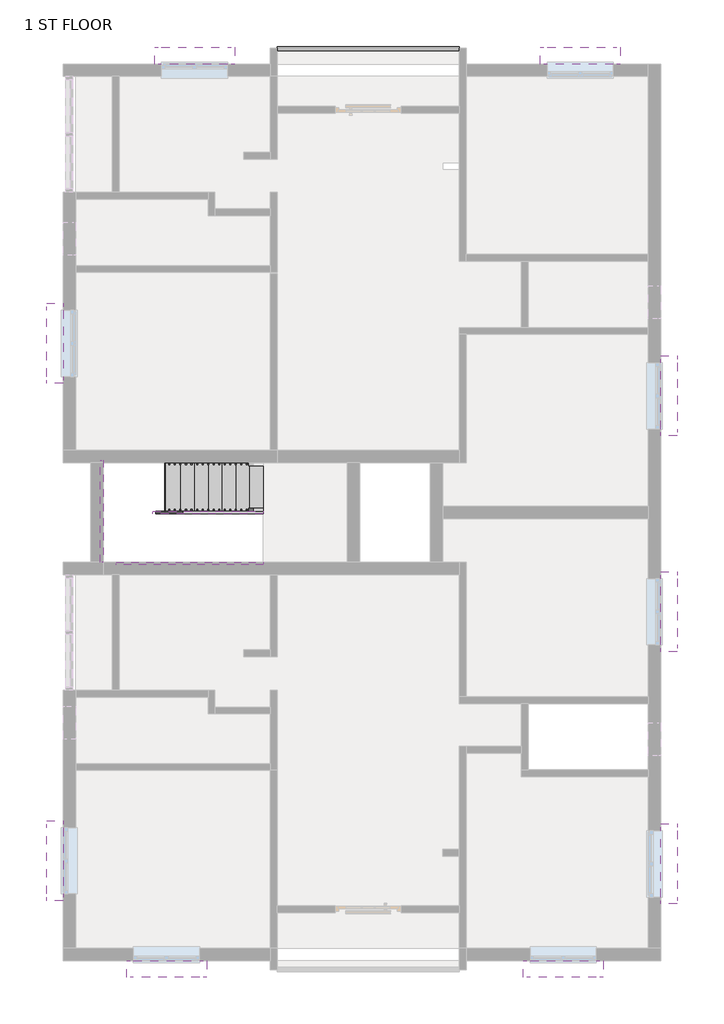
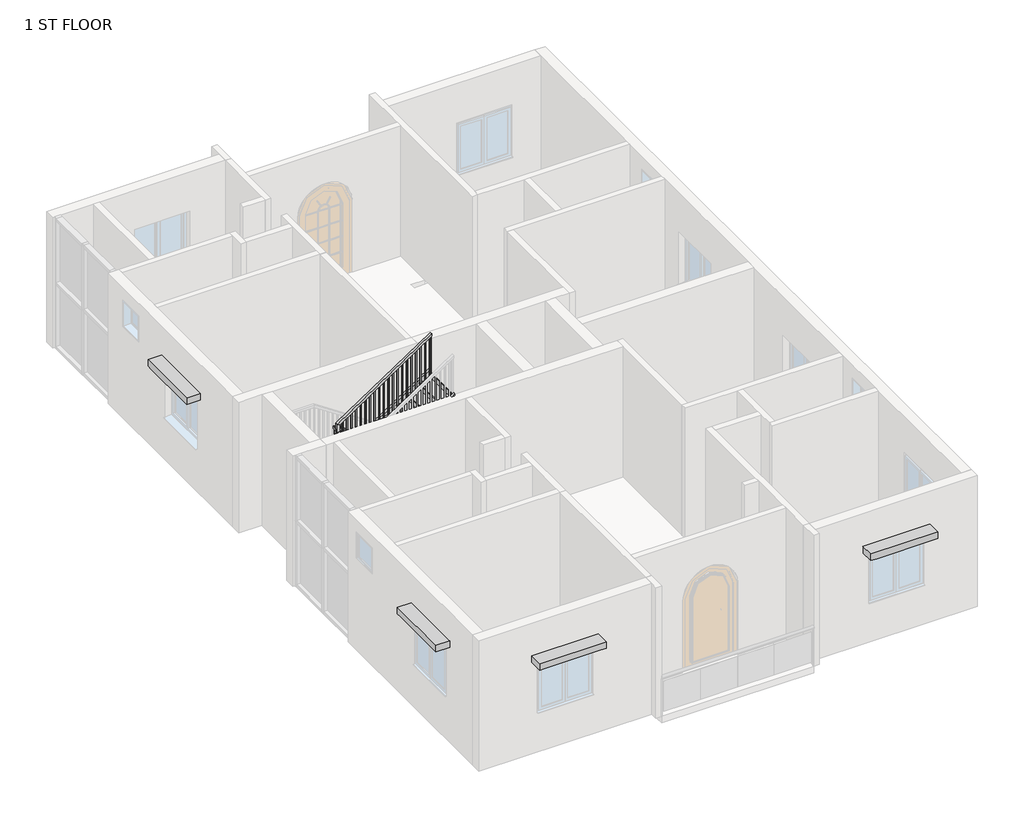
# One storey, part 4 of 4: 9 proxies, 5 members, 2 railings, 1 stair flight.
"""IFC4 building model written with IfcOpenShell, lengths in millimetres."""

from ifc_helpers import new_model, si_unit, point, frame, origin, place, context, project, spatial, polyline, ellipse_curve, trimmed, outline, extrude, faceted_brep, transform, mapped, element, save
from ifc_brep_helpers import plane_surface, extruded_surface, advanced_brep
from components import generic_models_11_generic_models_11_d301a5e8, generic_models_21_generic_models_21_87948dc1, generic_models_36_generic_models_36_9c63594f, generic_models_1_generic_models_1_fbb7ad13, stair_flight_02872950

model = new_model("IFC4")

# Units and contexts
model_context = context("Model", 3, world=origin())
ifc_project = project(units=[si_unit("LENGTHUNIT", "METRE", prefix="MILLI")], contexts=[model_context])

# Site, building, storey
site = spatial("IfcSite", under=ifc_project)
building = spatial("IfcBuilding", under=site)
storey = spatial("IfcBuildingStorey", under=building, Name="1 ST FLOOR", Elevation=6096.0)

# Proxies
placement = place(None, origin())
generic_models_11_generic_models_11_shape = generic_models_11_generic_models_11_d301a5e8(model_context)
element("IfcBuildingElementProxy", 1, Name="Generic Models 17 : Generic Models 11", ObjectType="Generic Models 17 : Generic Models 11", at=placement, inside=storey, context=model_context, shape_type="MappedRepresentation", body=[
    mapped(generic_models_11_generic_models_11_shape, transform((0.0, 0.0, -9144.0), x_axis=(1.0, 0.0, 0.0), y_axis=(0.0, 1.0, 0.0), z_axis=(0.0, 0.0, 1.0))),
])
element("IfcBuildingElementProxy", 2, Name="Generic Models 18 : Generic Models 11", ObjectType="Generic Models 18 : Generic Models 11", at=placement, inside=storey, context=model_context, shape_type="MappedRepresentation", body=[
    mapped(generic_models_11_generic_models_11_shape, transform((-7101.0359618, 0.0, -9144.0), x_axis=(1.0, 0.0, 0.0), y_axis=(0.0, 1.0, 0.0), z_axis=(0.0, 0.0, 1.0))),
])
generic_models_21_generic_models_21_shape = generic_models_21_generic_models_21_87948dc1(model_context)
element("IfcBuildingElementProxy", 3, Name="Generic Models 30 : Generic Models 21", ObjectType="Generic Models 30 : Generic Models 21", at=placement, inside=storey, context=model_context, shape_type="MappedRepresentation", body=[
    mapped(generic_models_21_generic_models_21_shape, transform((0.0, 0.0, -9144.0), x_axis=(1.0, 0.0, 0.0), y_axis=(0.0, 1.0, 0.0), z_axis=(0.0, 0.0, 1.0))),
])
element("IfcBuildingElementProxy", 4, Name="Generic Models 31 : Generic Models 21", ObjectType="Generic Models 31 : Generic Models 21", at=placement, inside=storey, context=model_context, shape_type="MappedRepresentation", body=[
    mapped(generic_models_21_generic_models_21_shape, transform((0.0, 4641.85, -9229.6), x_axis=(1.0, 0.0, 0.0), y_axis=(0.0, 1.0, 0.0), z_axis=(0.0, 0.0, 1.0))),
])
element("IfcBuildingElementProxy", 5, Name="Generic Models 32 : Generic Models 21", ObjectType="Generic Models 32 : Generic Models 21", at=placement, inside=storey, context=model_context, shape_type="MappedRepresentation", body=[
    mapped(generic_models_21_generic_models_21_shape, transform((0.0, 8616.95, -9229.6), x_axis=(1.0, 0.0, 0.0), y_axis=(0.0, 1.0, 0.0), z_axis=(0.0, 0.0, 1.0))),
])
generic_models_36_generic_models_36_shape = generic_models_36_generic_models_36_9c63594f(model_context)
element("IfcBuildingElementProxy", 6, Name="Generic Models 42 : Generic Models 36", ObjectType="Generic Models 42 : Generic Models 36", at=placement, inside=storey, context=model_context, shape_type="MappedRepresentation", body=[
    mapped(generic_models_36_generic_models_36_shape, transform((0.0, 0.0, -9144.0), x_axis=(1.0, 0.0, 0.0), y_axis=(0.0, 1.0, 0.0), z_axis=(0.0, 0.0, 1.0))),
])
element("IfcBuildingElementProxy", 7, Name="Generic Models 43 : Generic Models 36", ObjectType="Generic Models 43 : Generic Models 36", at=placement, inside=storey, context=model_context, shape_type="MappedRepresentation", body=[
    mapped(generic_models_36_generic_models_36_shape, transform((0.0, -9525.0, -9144.0), x_axis=(1.0, 0.0, 0.0), y_axis=(0.0, 1.0, 0.0), z_axis=(0.0, 0.0, 1.0))),
])
generic_models_1_generic_models_1_shape = generic_models_1_generic_models_1_fbb7ad13(model_context)
element("IfcBuildingElementProxy", 8, Name="Generic Models 7 : Generic Models 1", ObjectType="Generic Models 7 : Generic Models 1", at=placement, inside=storey, context=model_context, shape_type="MappedRepresentation", body=[
    mapped(generic_models_1_generic_models_1_shape, transform((0.0, 0.0, -9144.0), x_axis=(1.0, 0.0, 0.0), y_axis=(0.0, 1.0, 0.0), z_axis=(0.0, 0.0, 1.0))),
])
element("IfcBuildingElementProxy", 9, Name="Generic Models 8 : Generic Models 1", ObjectType="Generic Models 8 : Generic Models 1", at=placement, inside=storey, context=model_context, shape_type="MappedRepresentation", body=[
    mapped(generic_models_1_generic_models_1_shape, transform((7304.0875, 0.0, -9144.0), x_axis=(1.0, 0.0, 0.0), y_axis=(0.0, 1.0, 0.0), z_axis=(0.0, 0.0, 1.0))),
])

# Members
element("IfcMember", 10, ObjectType="Stringer - 2\" Width", at=placement, inside=storey, context=model_context, shape_type="SweptSolid", body=[
    extrude(outline(polyline([(6096.0, -2748.0012202), (6314.0398409, -2748.0012202), (7634.8398409, -4729.2012202), (7268.5158313, -4729.2012202), (6096.0, -2970.4274732), (6096.0, -2748.0012202)])), frame((0.0, 4990.8309003, 0.0), z_axis=(0.0, 1.0, 0.0), x_axis=(0.0, 0.0, 1.0)), (0.0, 0.0, 1.0), 50.8),
])
element("IfcMember", 11, ObjectType="Stringer - 2\" Width", at=placement, inside=storey, context=model_context, shape_type="SweptSolid", body=[
    extrude(outline(polyline([(7838.0398409, -4780.0012202), (7471.7158313, -4780.0012202), (8826.382498, -2748.0012202), (9192.7065076, -2748.0012202), (7838.0398409, -4780.0012202)])), frame((0.0, 4990.8309003, 0.0), z_axis=(0.0, 1.0, 0.0), x_axis=(0.0, 0.0, 1.0)), (0.0, 0.0, 1.0), 50.8),
])
element("IfcMember", 12, ObjectType="Stringer - 2\" Width", at=placement, inside=storey, context=model_context, shape_type="SweptSolid", body=[
    extrude(outline(polyline([(6096.0, -2748.0012202), (6314.0398409, -2748.0012202), (7696.2, -4821.2414588), (7696.2, -5370.7274732), (6096.0, -2970.4274732), (6096.0, -2748.0012202)])), frame((0.0, 5930.6309003, 0.0), z_axis=(0.0, 1.0, 0.0), x_axis=(0.0, 0.0, 1.0)), (0.0, 0.0, 1.0), 50.8),
])
element("IfcMember", 13, ObjectType="Stringer - 2\" Width", at=placement, inside=storey, context=model_context, shape_type="SweptSolid", body=[
    extrude(outline(polyline([(-5745.2012202, 5981.4309003), (-5694.4012202, 5981.4309003), (-5694.4012202, 4101.8309003), (-5745.2012202, 4101.8309003), (-5745.2012202, 5981.4309003)])), frame((0.0, 0.0, 7391.4), z_axis=(0.0, 0.0, 1.0), x_axis=(1.0, 0.0, 0.0)), (0.0, 0.0, 1.0), 304.8),
])
element("IfcMember", 14, ObjectType="Stringer - 2\" Width", at=placement, inside=storey, context=model_context, shape_type="SweptSolid", body=[
    extrude(outline(polyline([(7391.4, -4900.4749672), (8826.382498, -2748.0012202), (9192.7065076, -2748.0012202), (7391.4, -5449.9609815), (7391.4, -4900.4749672)])), frame((0.0, 4051.0309003, 0.0), z_axis=(0.0, 1.0, 0.0), x_axis=(0.0, 0.0, 1.0)), (0.0, 0.0, 1.0), 50.8),
])

# Railings
element("IfcRailing", 15, ObjectType="Glass Panel - Bottom Fill 2", at=placement, inside=storey, context=model_context, shape_type="SolidModel", body=[
    advanced_brep(
    [(-2494.0012202, 13593.7910566, 7010.4), (-2494.0012202, 13517.5910566, 7010.4), (858.7987798, 13593.7910566, 7010.4), (858.7987798, 13517.5910566, 7010.4)],
    [
        (0, 1, ellipse_curve(frame((-2494.0012202, 13555.6910566, 7010.4), z_axis=(-1.0, 0.0, 0.0), x_axis=(0.0, -1.0, 0.0)), 38.1, 28.575)),
        (1, 0, ellipse_curve(frame((-2494.0012202, 13555.6910566, 7010.4), z_axis=(-1.0, 0.0, 0.0), x_axis=(0.0, -1.0, 0.0)), 38.1, 28.575)),
        (2, 3, ellipse_curve(frame((858.7987798, 13555.6910566, 7010.4), z_axis=(1.0, 0.0, 0.0), x_axis=(0.0, -1.0, 0.0)), 38.1, 28.575)),
        (3, 2, ellipse_curve(frame((858.7987798, 13555.6910566, 7010.4), z_axis=(1.0, 0.0, 0.0), x_axis=(0.0, -1.0, 0.0)), 38.1, 28.575)),
        (0, 2),
        (3, 1),
    ],
    [
        plane_surface(frame((-2494.0012202, 13555.6910566, 7010.4), z_axis=(-1.0, 0.0, 0.0), x_axis=(0.0, 1.0, 0.0))),
        plane_surface(frame((858.7987798, 13555.6910566, 7010.4), z_axis=(1.0, 0.0, 0.0), x_axis=(0.0, 1.0, 0.0))),
        extruded_surface(trimmed(ellipse_curve(frame((858.7987798, 13555.6910566, 7010.4), z_axis=(-1.0, 0.0, 0.0), x_axis=(0.0, -1.0, 0.0)), 38.1, 28.575), [point((858.7987798, 13593.7910566, 7010.4))], [point((858.7987798, 13517.5910566, 7010.4))], True, "CARTESIAN"), (-3352.7999999999997, 0.0, 0.0), 3352.7999999999997),
        extruded_surface(trimmed(ellipse_curve(frame((858.7987798, 13555.6910566, 7010.4), z_axis=(-1.0, 0.0, 0.0), x_axis=(0.0, -1.0, 0.0)), 38.1, 28.575), [point((858.7987798, 13517.5910566, 7010.4))], [point((858.7987798, 13593.7910566, 7010.4))], True, "CARTESIAN"), (-3352.7999999999997, 0.0, 0.0), 3352.7999999999997),
    ],
    [
        (0, [[1, 2]]),
        (1, [[3, 4]]),
        (2, [[-1, 5, -4, 6]]),
        (3, [[-2, -6, -3, -5]]),
    ],
),
    extrude(outline(polyline([(-4.8012202, 13562.2262136), (807.9987798, 13562.2262136), (807.9987798, 13555.8762136), (-4.8012202, 13555.8762136), (-4.8012202, 13562.2262136)])), frame((0.0, 0.0, 6197.6), z_axis=(0.0, 0.0, 1.0), x_axis=(1.0, 0.0, 0.0)), (0.0, 0.0, 1.0), 711.2),
    extrude(outline(polyline([(-817.6012202, 13562.2262136), (-4.8012202, 13562.2262136), (-4.8012202, 13555.8762136), (-817.6012202, 13555.8762136), (-817.6012202, 13562.2262136)])), frame((0.0, 0.0, 6197.6), z_axis=(0.0, 0.0, 1.0), x_axis=(1.0, 0.0, 0.0)), (0.0, 0.0, 1.0), 711.2),
    extrude(outline(polyline([(-1630.4012202, 13562.2262136), (-817.6012202, 13562.2262136), (-817.6012202, 13555.8762136), (-1630.4012202, 13555.8762136), (-1630.4012202, 13562.2262136)])), frame((0.0, 0.0, 6197.6), z_axis=(0.0, 0.0, 1.0), x_axis=(1.0, 0.0, 0.0)), (0.0, 0.0, 1.0), 711.2),
    extrude(outline(polyline([(-2443.2012202, 13562.2262136), (-1630.4012202, 13562.2262136), (-1630.4012202, 13555.8762136), (-2443.2012202, 13555.8762136), (-2443.2012202, 13562.2262136)])), frame((0.0, 0.0, 6197.6), z_axis=(0.0, 0.0, 1.0), x_axis=(1.0, 0.0, 0.0)), (0.0, 0.0, 1.0), 711.2),
    extrude(outline(polyline([(846.0987798, 13546.1660566), (846.0987798, 13565.2160566), (865.1487798, 13565.2160566), (865.1487798, 13546.1660566), (846.0987798, 13546.1660566)])), frame((0.0, 0.0, 6096.0), z_axis=(0.0, 0.0, 1.0), x_axis=(1.0, 0.0, 0.0)), (0.0, 0.0, 1.0), 885.825),
    extrude(outline(polyline([(-2500.3512202, 13546.1660566), (-2500.3512202, 13565.2160566), (-2481.3012202, 13565.2160566), (-2481.3012202, 13546.1660566), (-2500.3512202, 13546.1660566)])), frame((0.0, 0.0, 6096.0), z_axis=(0.0, 0.0, 1.0), x_axis=(1.0, 0.0, 0.0)), (0.0, 0.0, 1.0), 885.825),
])
element("IfcRailing", 16, ObjectType="Handrail - Rectangular", at=placement, inside=storey, context=model_context, shape_type="SolidModel", body=[
    faceted_brep([(-2748.0012202, 5041.6309003, 7179.7333333), (-2748.0012202, 5041.6309003, 7118.6793317), (-2748.0012202, 5092.4309003, 7118.6793317), (-2748.0012202, 5092.4309003, 7179.7333333), (-4703.8012202, 5041.6309003, 8483.6), (-4754.6012202, 5041.6309003, 8456.4126651), (-4754.6012202, 5092.4309003, 8456.4126651), (-4703.8012202, 5092.4309003, 8483.6), (-4703.8012202, 5041.6309003, 8534.4), (-4754.6012202, 5041.6309003, 8483.6), (-4754.6012202, 5092.4309003, 8483.6), (-4703.8012202, 5092.4309003, 8534.4), (-4780.0012202, 5041.6309003, 8534.4), (-4780.0012202, 5041.6309003, 8483.6), (-4830.8012202, 5092.4309003, 8483.6), (-4830.8012202, 5092.4309003, 8534.4), (-4780.0012202, 4990.8309003, 8534.4), (-4830.8012202, 4990.8309003, 8534.4), (-4830.8012202, 4940.0309003, 8483.6), (-4780.0012202, 4940.0309003, 8483.6)], [[[0, 1, 2, 3]], [[1, 0, 4, 5]], [[2, 1, 5, 6]], [[3, 2, 6, 7]], [[0, 3, 7, 4]], [[5, 4, 8, 9]], [[6, 5, 9, 10]], [[7, 6, 10, 11]], [[4, 7, 11, 8]], [[9, 8, 12, 13]], [[10, 9, 13, 14]], [[11, 10, 14, 15]], [[8, 11, 15, 12]], [[16, 17, 18, 19]], [[13, 12, 16, 19]], [[14, 13, 19, 18]], [[15, 14, 18, 17]], [[12, 15, 17, 16]]]),
    faceted_brep([(-4780.0012202, 4990.8309003, 8534.4), (-4780.0012202, 4940.0309003, 8483.6), (-4830.8012202, 4940.0309003, 8483.6), (-4830.8012202, 4990.8309003, 8534.4), (-4780.0012202, 4990.8309003, 8642.6793317), (-4830.8012202, 4990.8309003, 8669.8666667), (-4830.8012202, 4940.0309003, 8669.8666667), (-4780.0012202, 4940.0309003, 8642.6793317)], [[[0, 1, 2, 3]], [[4, 5, 6, 7]], [[1, 0, 4, 7]], [[2, 1, 7, 6]], [[3, 2, 6, 5]], [[0, 3, 5, 4]]]),
    faceted_brep([(-4830.8012202, 4990.8309003, 8669.8666667), (-4780.0012202, 4990.8309003, 8642.6793317), (-4780.0012202, 4940.0309003, 8642.6793317), (-4830.8012202, 4940.0309003, 8669.8666667), (-2748.0012202, 4990.8309003, 10058.4), (-2748.0012202, 4940.0309003, 10058.4), (-2748.0012202, 4940.0309003, 9997.3459984), (-2748.0012202, 4990.8309003, 9997.3459984)], [[[0, 1, 2, 3]], [[4, 5, 6, 7]], [[1, 0, 4, 7]], [[2, 1, 7, 6]], [[3, 2, 6, 5]], [[0, 3, 5, 4]]]),
    extrude(outline(polyline([(9974.0626651, -2782.9262202), (8974.6666667, -2782.9262202), (8974.6666667, -2763.8762202), (9986.7626651, -2763.8762202), (9974.0626651, -2782.9262202)])), frame((0.0, 4955.9059003, 0.0), z_axis=(0.0, 1.0, 0.0), x_axis=(0.0, 0.0, 1.0)), (0.0, 0.0, 1.0), 19.05),
    extrude(outline(polyline([(9906.3293317, -2884.5262202), (8974.6666667, -2884.5262202), (8974.6666667, -2865.4762202), (9919.0293317, -2865.4762202), (9906.3293317, -2884.5262202)])), frame((0.0, 4955.9059003, 0.0), z_axis=(0.0, 1.0, 0.0), x_axis=(0.0, 0.0, 1.0)), (0.0, 0.0, 1.0), 19.05),
    extrude(outline(polyline([(9838.5959984, -2986.1262202), (8974.6666667, -2986.1262202), (8974.6666667, -2967.0762202), (9851.2959984, -2967.0762202), (9838.5959984, -2986.1262202)])), frame((0.0, 4955.9059003, 0.0), z_axis=(0.0, 1.0, 0.0), x_axis=(0.0, 0.0, 1.0)), (0.0, 0.0, 1.0), 19.05),
    extrude(outline(polyline([(9770.8626651, -3087.7262202), (8805.3333333, -3087.7262202), (8805.3333333, -3068.6762202), (9783.5626651, -3068.6762202), (9770.8626651, -3087.7262202)])), frame((0.0, 4955.9059003, 0.0), z_axis=(0.0, 1.0, 0.0), x_axis=(0.0, 0.0, 1.0)), (0.0, 0.0, 1.0), 19.05),
    extrude(outline(polyline([(9703.1293317, -3189.3262202), (8805.3333333, -3189.3262202), (8805.3333333, -3170.2762202), (9715.8293317, -3170.2762202), (9703.1293317, -3189.3262202)])), frame((0.0, 4955.9059003, 0.0), z_axis=(0.0, 1.0, 0.0), x_axis=(0.0, 0.0, 1.0)), (0.0, 0.0, 1.0), 19.05),
    extrude(outline(polyline([(9635.3959984, -3290.9262202), (8636.0, -3290.9262202), (8636.0, -3271.8762202), (9648.0959984, -3271.8762202), (9635.3959984, -3290.9262202)])), frame((0.0, 4955.9059003, 0.0), z_axis=(0.0, 1.0, 0.0), x_axis=(0.0, 0.0, 1.0)), (0.0, 0.0, 1.0), 19.05),
    extrude(outline(polyline([(9567.6626651, -3392.5262202), (8636.0, -3392.5262202), (8636.0, -3373.4762202), (9580.3626651, -3373.4762202), (9567.6626651, -3392.5262202)])), frame((0.0, 4955.9059003, 0.0), z_axis=(0.0, 1.0, 0.0), x_axis=(0.0, 0.0, 1.0)), (0.0, 0.0, 1.0), 19.05),
    extrude(outline(polyline([(9499.9293317, -3494.1262202), (8636.0, -3494.1262202), (8636.0, -3475.0762202), (9512.6293317, -3475.0762202), (9499.9293317, -3494.1262202)])), frame((0.0, 4955.9059003, 0.0), z_axis=(0.0, 1.0, 0.0), x_axis=(0.0, 0.0, 1.0)), (0.0, 0.0, 1.0), 19.05),
    extrude(outline(polyline([(9432.1959984, -3595.7262202), (8466.6666667, -3595.7262202), (8466.6666667, -3576.6762202), (9444.8959984, -3576.6762202), (9432.1959984, -3595.7262202)])), frame((0.0, 4955.9059003, 0.0), z_axis=(0.0, 1.0, 0.0), x_axis=(0.0, 0.0, 1.0)), (0.0, 0.0, 1.0), 19.05),
    extrude(outline(polyline([(9364.4626651, -3697.3262202), (8466.6666667, -3697.3262202), (8466.6666667, -3678.2762202), (9377.1626651, -3678.2762202), (9364.4626651, -3697.3262202)])), frame((0.0, 4955.9059003, 0.0), z_axis=(0.0, 1.0, 0.0), x_axis=(0.0, 0.0, 1.0)), (0.0, 0.0, 1.0), 19.05),
    extrude(outline(polyline([(9296.7293317, -3798.9262202), (8297.3333333, -3798.9262202), (8297.3333333, -3779.8762202), (9309.4293317, -3779.8762202), (9296.7293317, -3798.9262202)])), frame((0.0, 4955.9059003, 0.0), z_axis=(0.0, 1.0, 0.0), x_axis=(0.0, 0.0, 1.0)), (0.0, 0.0, 1.0), 19.05),
    extrude(outline(polyline([(9228.9959984, -3900.5262202), (8297.3333333, -3900.5262202), (8297.3333333, -3881.4762202), (9241.6959984, -3881.4762202), (9228.9959984, -3900.5262202)])), frame((0.0, 4955.9059003, 0.0), z_axis=(0.0, 1.0, 0.0), x_axis=(0.0, 0.0, 1.0)), (0.0, 0.0, 1.0), 19.05),
    extrude(outline(polyline([(9161.2626651, -4002.1262202), (8297.3333333, -4002.1262202), (8297.3333333, -3983.0762202), (9173.9626651, -3983.0762202), (9161.2626651, -4002.1262202)])), frame((0.0, 4955.9059003, 0.0), z_axis=(0.0, 1.0, 0.0), x_axis=(0.0, 0.0, 1.0)), (0.0, 0.0, 1.0), 19.05),
    extrude(outline(polyline([(9093.5293317, -4103.7262202), (8128.0, -4103.7262202), (8128.0, -4084.6762202), (9106.2293317, -4084.6762202), (9093.5293317, -4103.7262202)])), frame((0.0, 4955.9059003, 0.0), z_axis=(0.0, 1.0, 0.0), x_axis=(0.0, 0.0, 1.0)), (0.0, 0.0, 1.0), 19.05),
    extrude(outline(polyline([(9025.7959984, -4205.3262202), (8128.0, -4205.3262202), (8128.0, -4186.2762202), (9038.4959984, -4186.2762202), (9025.7959984, -4205.3262202)])), frame((0.0, 4955.9059003, 0.0), z_axis=(0.0, 1.0, 0.0), x_axis=(0.0, 0.0, 1.0)), (0.0, 0.0, 1.0), 19.05),
    extrude(outline(polyline([(8958.0626651, -4306.9262202), (7958.6666667, -4306.9262202), (7958.6666667, -4287.8762202), (8970.7626651, -4287.8762202), (8958.0626651, -4306.9262202)])), frame((0.0, 4955.9059003, 0.0), z_axis=(0.0, 1.0, 0.0), x_axis=(0.0, 0.0, 1.0)), (0.0, 0.0, 1.0), 19.05),
    extrude(outline(polyline([(8890.3293317, -4408.5262202), (7958.6666667, -4408.5262202), (7958.6666667, -4389.4762202), (8903.0293317, -4389.4762202), (8890.3293317, -4408.5262202)])), frame((0.0, 4955.9059003, 0.0), z_axis=(0.0, 1.0, 0.0), x_axis=(0.0, 0.0, 1.0)), (0.0, 0.0, 1.0), 19.05),
    extrude(outline(polyline([(8822.5959984, -4510.1262202), (7958.6666667, -4510.1262202), (7958.6666667, -4491.0762202), (8835.2959984, -4491.0762202), (8822.5959984, -4510.1262202)])), frame((0.0, 4955.9059003, 0.0), z_axis=(0.0, 1.0, 0.0), x_axis=(0.0, 0.0, 1.0)), (0.0, 0.0, 1.0), 19.05),
    extrude(outline(polyline([(8754.8626651, -4611.7262202), (7789.3333333, -4611.7262202), (7789.3333333, -4592.6762202), (8767.5626651, -4592.6762202), (8754.8626651, -4611.7262202)])), frame((0.0, 4955.9059003, 0.0), z_axis=(0.0, 1.0, 0.0), x_axis=(0.0, 0.0, 1.0)), (0.0, 0.0, 1.0), 19.05),
    extrude(outline(polyline([(8687.1293317, -4713.3262202), (7789.3333333, -4713.3262202), (7789.3333333, -4694.2762202), (8699.8293317, -4694.2762202), (8687.1293317, -4713.3262202)])), frame((0.0, 4955.9059003, 0.0), z_axis=(0.0, 1.0, 0.0), x_axis=(0.0, 0.0, 1.0)), (0.0, 0.0, 1.0), 19.05),
    extrude(outline(polyline([(-4770.4762202, 5057.5059003), (-4789.5262202, 5057.5059003), (-4789.5262202, 5076.5559003), (-4770.4762202, 5076.5559003), (-4770.4762202, 5057.5059003)])), frame((0.0, 0.0, 7620.0), z_axis=(0.0, 0.0, 1.0), x_axis=(1.0, 0.0, 0.0)), (0.0, 0.0, 1.0), 863.6),
    extrude(outline(polyline([(8411.9626651, -4687.9262202), (7450.6666667, -4687.9262202), (7450.6666667, -4668.8762202), (8399.2626651, -4668.8762202), (8411.9626651, -4687.9262202)])), frame((0.0, 5057.5059003, 0.0), z_axis=(0.0, 1.0, 0.0), x_axis=(0.0, 0.0, 1.0)), (0.0, 0.0, 1.0), 19.05),
    extrude(outline(polyline([(8344.2293317, -4586.3262202), (7450.6666667, -4586.3262202), (7450.6666667, -4567.2762202), (8331.5293317, -4567.2762202), (8344.2293317, -4586.3262202)])), frame((0.0, 5057.5059003, 0.0), z_axis=(0.0, 1.0, 0.0), x_axis=(0.0, 0.0, 1.0)), (0.0, 0.0, 1.0), 19.05),
    extrude(outline(polyline([(8276.4959984, -4484.7262202), (7281.3333333, -4484.7262202), (7281.3333333, -4465.6762202), (8263.7959984, -4465.6762202), (8276.4959984, -4484.7262202)])), frame((0.0, 5057.5059003, 0.0), z_axis=(0.0, 1.0, 0.0), x_axis=(0.0, 0.0, 1.0)), (0.0, 0.0, 1.0), 19.05),
    extrude(outline(polyline([(8208.7626651, -4383.1262202), (7281.3333333, -4383.1262202), (7281.3333333, -4364.0762202), (8196.0626651, -4364.0762202), (8208.7626651, -4383.1262202)])), frame((0.0, 5057.5059003, 0.0), z_axis=(0.0, 1.0, 0.0), x_axis=(0.0, 0.0, 1.0)), (0.0, 0.0, 1.0), 19.05),
    extrude(outline(polyline([(8141.0293317, -4281.5262202), (7281.3333333, -4281.5262202), (7281.3333333, -4262.4762202), (8128.3293317, -4262.4762202), (8141.0293317, -4281.5262202)])), frame((0.0, 5057.5059003, 0.0), z_axis=(0.0, 1.0, 0.0), x_axis=(0.0, 0.0, 1.0)), (0.0, 0.0, 1.0), 19.05),
    extrude(outline(polyline([(8073.2959984, -4179.9262202), (7112.0, -4179.9262202), (7112.0, -4160.8762202), (8060.5959984, -4160.8762202), (8073.2959984, -4179.9262202)])), frame((0.0, 5057.5059003, 0.0), z_axis=(0.0, 1.0, 0.0), x_axis=(0.0, 0.0, 1.0)), (0.0, 0.0, 1.0), 19.05),
    extrude(outline(polyline([(8005.5626651, -4078.3262202), (7112.0, -4078.3262202), (7112.0, -4059.2762202), (7992.8626651, -4059.2762202), (8005.5626651, -4078.3262202)])), frame((0.0, 5057.5059003, 0.0), z_axis=(0.0, 1.0, 0.0), x_axis=(0.0, 0.0, 1.0)), (0.0, 0.0, 1.0), 19.05),
    extrude(outline(polyline([(7937.8293317, -3976.7262202), (6942.6666667, -3976.7262202), (6942.6666667, -3957.6762202), (7925.1293317, -3957.6762202), (7937.8293317, -3976.7262202)])), frame((0.0, 5057.5059003, 0.0), z_axis=(0.0, 1.0, 0.0), x_axis=(0.0, 0.0, 1.0)), (0.0, 0.0, 1.0), 19.05),
    extrude(outline(polyline([(7870.0959984, -3875.1262202), (6942.6666667, -3875.1262202), (6942.6666667, -3856.0762202), (7857.3959984, -3856.0762202), (7870.0959984, -3875.1262202)])), frame((0.0, 5057.5059003, 0.0), z_axis=(0.0, 1.0, 0.0), x_axis=(0.0, 0.0, 1.0)), (0.0, 0.0, 1.0), 19.05),
    extrude(outline(polyline([(7802.3626651, -3773.5262202), (6942.6666667, -3773.5262202), (6942.6666667, -3754.4762202), (7789.6626651, -3754.4762202), (7802.3626651, -3773.5262202)])), frame((0.0, 5057.5059003, 0.0), z_axis=(0.0, 1.0, 0.0), x_axis=(0.0, 0.0, 1.0)), (0.0, 0.0, 1.0), 19.05),
    extrude(outline(polyline([(7734.6293317, -3671.9262202), (6773.3333333, -3671.9262202), (6773.3333333, -3652.8762202), (7721.9293317, -3652.8762202), (7734.6293317, -3671.9262202)])), frame((0.0, 5057.5059003, 0.0), z_axis=(0.0, 1.0, 0.0), x_axis=(0.0, 0.0, 1.0)), (0.0, 0.0, 1.0), 19.05),
    extrude(outline(polyline([(7666.8959984, -3570.3262202), (6773.3333333, -3570.3262202), (6773.3333333, -3551.2762202), (7654.1959984, -3551.2762202), (7666.8959984, -3570.3262202)])), frame((0.0, 5057.5059003, 0.0), z_axis=(0.0, 1.0, 0.0), x_axis=(0.0, 0.0, 1.0)), (0.0, 0.0, 1.0), 19.05),
    extrude(outline(polyline([(7599.1626651, -3468.7262202), (6604.0, -3468.7262202), (6604.0, -3449.6762202), (7586.4626651, -3449.6762202), (7599.1626651, -3468.7262202)])), frame((0.0, 5057.5059003, 0.0), z_axis=(0.0, 1.0, 0.0), x_axis=(0.0, 0.0, 1.0)), (0.0, 0.0, 1.0), 19.05),
    extrude(outline(polyline([(7531.4293317, -3367.1262202), (6604.0, -3367.1262202), (6604.0, -3348.0762202), (7518.7293317, -3348.0762202), (7531.4293317, -3367.1262202)])), frame((0.0, 5057.5059003, 0.0), z_axis=(0.0, 1.0, 0.0), x_axis=(0.0, 0.0, 1.0)), (0.0, 0.0, 1.0), 19.05),
    extrude(outline(polyline([(7463.6959984, -3265.5262202), (6604.0, -3265.5262202), (6604.0, -3246.4762202), (7450.9959984, -3246.4762202), (7463.6959984, -3265.5262202)])), frame((0.0, 5057.5059003, 0.0), z_axis=(0.0, 1.0, 0.0), x_axis=(0.0, 0.0, 1.0)), (0.0, 0.0, 1.0), 19.05),
    extrude(outline(polyline([(7395.9626651, -3163.9262202), (6434.6666667, -3163.9262202), (6434.6666667, -3144.8762202), (7383.2626651, -3144.8762202), (7395.9626651, -3163.9262202)])), frame((0.0, 5057.5059003, 0.0), z_axis=(0.0, 1.0, 0.0), x_axis=(0.0, 0.0, 1.0)), (0.0, 0.0, 1.0), 19.05),
    extrude(outline(polyline([(7328.2293317, -3062.3262202), (6434.6666667, -3062.3262202), (6434.6666667, -3043.2762202), (7315.5293317, -3043.2762202), (7328.2293317, -3062.3262202)])), frame((0.0, 5057.5059003, 0.0), z_axis=(0.0, 1.0, 0.0), x_axis=(0.0, 0.0, 1.0)), (0.0, 0.0, 1.0), 19.05),
    extrude(outline(polyline([(7260.4959984, -2960.7262202), (6265.3333333, -2960.7262202), (6265.3333333, -2941.6762202), (7247.7959984, -2941.6762202), (7260.4959984, -2960.7262202)])), frame((0.0, 5057.5059003, 0.0), z_axis=(0.0, 1.0, 0.0), x_axis=(0.0, 0.0, 1.0)), (0.0, 0.0, 1.0), 19.05),
    extrude(outline(polyline([(7192.7626651, -2859.1262202), (6265.3333333, -2859.1262202), (6265.3333333, -2840.0762202), (7180.0626651, -2840.0762202), (7192.7626651, -2859.1262202)])), frame((0.0, 5057.5059003, 0.0), z_axis=(0.0, 1.0, 0.0), x_axis=(0.0, 0.0, 1.0)), (0.0, 0.0, 1.0), 19.05),
    extrude(outline(polyline([(-4795.8762202, 4974.9559003), (-4795.8762202, 4955.9059003), (-4814.9262202, 4955.9059003), (-4814.9262202, 4974.9559003), (-4795.8762202, 4974.9559003)])), frame((0.0, 0.0, 7620.0), z_axis=(0.0, 0.0, 1.0), x_axis=(1.0, 0.0, 0.0)), (0.0, 0.0, 1.0), 863.6),
    extrude(outline(polyline([(-4795.8762202, 5057.5059003), (-4814.9262202, 5057.5059003), (-4814.9262202, 5076.5559003), (-4795.8762202, 5076.5559003), (-4795.8762202, 5057.5059003)])), frame((0.0, 0.0, 7620.0), z_axis=(0.0, 0.0, 1.0), x_axis=(1.0, 0.0, 0.0)), (0.0, 0.0, 1.0), 863.6),
    extrude(outline(polyline([(9984.6459984, -2767.0512202), (8974.6666667, -2767.0512202), (8974.6666667, -2748.0012202), (9997.3459984, -2748.0012202), (9984.6459984, -2767.0512202)])), frame((0.0, 4955.9059003, 0.0), z_axis=(0.0, 1.0, 0.0), x_axis=(0.0, 0.0, 1.0)), (0.0, 0.0, 1.0), 19.05),
    extrude(outline(polyline([(7131.3793317, -2767.0512202), (6265.3333333, -2767.0512202), (6265.3333333, -2748.0012202), (7118.6793317, -2748.0012202), (7131.3793317, -2767.0512202)])), frame((0.0, 5057.5059003, 0.0), z_axis=(0.0, 1.0, 0.0), x_axis=(0.0, 0.0, 1.0)), (0.0, 0.0, 1.0), 19.05),
])

# Stair flight
stair_flight_shape = stair_flight_02872950(model_context)
element("IfcStairFlight", 17, ObjectType="2\" Tread 1\" Nosing 1/4\" Riser", at=placement, inside=storey, context=model_context, shape_type="MappedRepresentation", body=[
    mapped(stair_flight_shape, transform((0.0, 0.0, 0.0), x_axis=(1.0, 0.0, 0.0), y_axis=(0.0, 1.0, 0.0), z_axis=(0.0, 0.0, 1.0))),
])

save(model, "model.ifc")

# Revit data of these elements
# Type "Glass Panel - Bottom Fill 2"
#   Assembly Code = "C2010400"
#   built-in parameter 1008612 = 0.0416667 (stored number, unit not read)
#   built-in parameter 1008611 = 0.0416667 (stored number, unit not read)
#   built-in parameter 1008609 = 0.333333 (stored number, unit not read)
#   built-in parameter 1008604 = 0.166667 (stored number, unit not read)
#   built-in parameter 1008603 = 0.166667 (stored number, unit not read)
#   Railing Height = 3' - 0"
#   built-in parameter 1008630 = 2
#   built-in parameter 1008610 = 2
#   built-in parameter 1008618 = Baluster - Square : 3/4"
# Type "Handrail - Rectangular"
#   Assembly Code = "C2010400"
#   built-in parameter 1008612 = 0.0416667 (stored number, unit not read)
#   built-in parameter 1008611 = 0.0416667 (stored number, unit not read)
#   built-in parameter 1008609 = 0.333333 (stored number, unit not read)
#   built-in parameter 1008604 = 0.166667 (stored number, unit not read)
#   built-in parameter 1008603 = 0.166667 (stored number, unit not read)
#   Railing Height = 3' - 0"
#   built-in parameter 1008630 = 2
#   built-in parameter 1008610 = 2
#   built-in parameter 1008618 = Baluster - Square : 3/4"
# Element 1 (IfcBuildingElementProxy, "Generic Models 17 : Generic Models 11")
#   Phase Created = New Construction
#   Materials on its faces: "white"
# Element 2 (IfcBuildingElementProxy, "Generic Models 18 : Generic Models 11")
#   Phase Created = New Construction
#   Materials on its faces: "white"
# Element 3 (IfcBuildingElementProxy, "Generic Models 30 : Generic Models 21")
#   Phase Created = New Construction
#   Materials on its faces: "white"
# Element 4 (IfcBuildingElementProxy, "Generic Models 31 : Generic Models 21")
#   Phase Created = New Construction
#   Materials on its faces: "white"
# Element 5 (IfcBuildingElementProxy, "Generic Models 32 : Generic Models 21")
#   Phase Created = New Construction
#   Materials on its faces: "white"
# Element 6 (IfcBuildingElementProxy, "Generic Models 42 : Generic Models 36")
#   Phase Created = New Construction
#   Materials on its faces: "white"
# Element 7 (IfcBuildingElementProxy, "Generic Models 43 : Generic Models 36")
#   Phase Created = New Construction
#   Materials on its faces: "white"
# Element 8 (IfcBuildingElementProxy, "Generic Models 7 : Generic Models 1")
#   Phase Created = New Construction
#   Materials on its faces: "white"
# Element 9 (IfcBuildingElementProxy, "Generic Models 8 : Generic Models 1")
#   Phase Created = New Construction
#   Materials on its faces: "white"
# Elements 10, 11, 12, 13, 14 (IfcMember, "Stringer - 2\" Width")
#   Phase Created = New Construction
# Element 15 (IfcRailing, "Glass Panel - Bottom Fill 2")
#   Phase Created = New Construction
#   Materials on its faces: "Glass"
# Element 16 (IfcRailing, "Handrail - Rectangular")
#   Phase Created = New Construction
# Element 17 (IfcStairFlight, "2\" Tread 1\" Nosing 1/4\" Riser")
#   Phase Created = New Construction
# Materials
#   "white": class "Generic", colour RGB 120 120 120, transparency 0, Cost = 0
#   "Glass": class "Glass", colour RGB 0 128 192, transparency 0.75, Description = "Soda Lime Glass", Cost = 0
